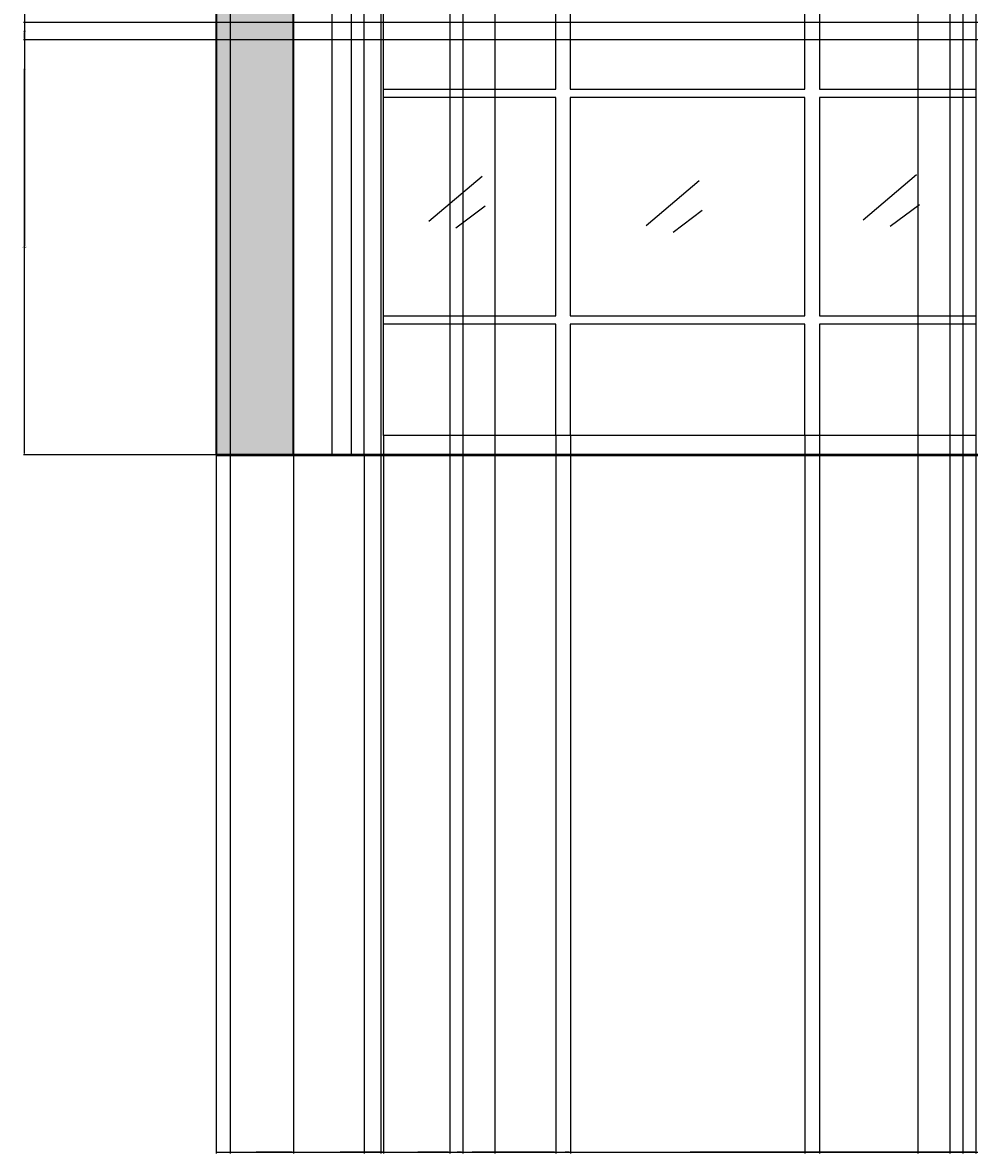
# Model space of a CAD drawing. Units: inches. Extents: x -13 to 630, y -103 to 275.
# Tile 1 of 9: x -13 to 134, y -103 to 72. Entities that reach past the tile are written whole.
import ezdxf

# ---------------------------------------------------------------- set-up
doc = ezdxf.new("R2010")
doc.units = ezdxf.units.IN
doc.header["$MEASUREMENT"] = 0
for name, color, linetype, lineweight in [('A-ANNO-DIMS', 2, 'Continuous', 18), ('A-ELEV', 7, 'Continuous', 35), ('A-ELEV-GRND', 7, 'Continuous', 50), ('A-ELEV-PATT', 8, 'Continuous', 13), ('A-GLAZ', 4, 'Continuous', 25)]:
    doc.layers.add(name, color=color, linetype=linetype, lineweight=lineweight)
doc.styles.get("Standard").update_dxf_attribs({"font": 'arial.ttf'})
doc.dimstyles.get("Standard").update_dxf_attribs({"dimtxt": 0.18, "dimasz": 0.18, "dimexe": 0.18, "dimexo": 0.0625, "dimgap": 0.09, "dimtad": 0, "dimtih": 1, "dimtoh": 1, "dimdec": 4, "dimzin": 0, "dimdsep": 46, "dimtxsty": 'Standard', "dimcen": 0.09, "dimadec": 0, "dimazin": 0, "dimtfac": 1, "dimtdec": 4, "dimtofl": 0, "dimtmove": 0, "dimatfit": 3, "dimfxl": 1, "dimtolj": 1, "dimtzin": 0, "dimarcsym": 0})

# ---------------------------------------------------------------- blocks, each defined once
blk = doc.blocks.new('WIN-GROUND')
for points in [[(0, 0), (0, 102), (108, 102), (108, 0)], [(3, 0), (3, 99), (105, 99), (105, 0)], [(5, 0), (5, 97), (103, 97), (103, 0)], [(34.74, 56.82), (34.74, 73.49), (37, 73.49), (37, 56.82)], [(73.43, 56.82), (73.43, 73.49), (75.7, 73.49), (75.7, 56.82)], [(34.74, 55.51), (8, 55.51), (8, 56.82), (34.74, 56.82)], [(37, 56.82), (73.43, 56.82)], [(75.7, 56.82), (100, 56.82), (100, 55.51), (75.7, 55.51)], [(34.74, 21.58), (34.74, 55.51)], [(37, 55.51), (37, 21.58)], [(73.43, 55.51), (37, 55.51)], [(73.43, 21.58), (73.43, 55.51)], [(75.7, 55.51), (75.7, 21.58)], [(34.74, 20.27), (8, 20.27), (8, 21.58), (34.74, 21.58)], [(37, 21.58), (73.43, 21.58)], [(75.7, 21.58), (100, 21.58), (100, 20.27), (75.7, 20.27)], [(37, 20.27), (37, 3), (34.74, 3), (34.74, 20.27)], [(73.43, 20.27), (37, 20.27)], [(75.7, 20.27), (75.7, 3), (73.43, 3), (73.43, 20.27)]]:
    blk.add_lwpolyline(points)
for points in [[(5, 97), (103, 97), (103, 76.49), (5, 76.49)], [(5, 76.49), (103, 76.49), (103, 0), (5, 0)], [(8, 73.49), (100, 73.49), (100, 3), (8, 3)]]:
    blk.add_lwpolyline(points, close=True)
blk = doc.blocks.new('GLAZ-MARK')
for p, q in [((0, 1.02), (8.26, 8.03)), ((4.19, 0), (8.71, 3.39))]:
    blk.add_line(p, q)
blk = doc.blocks.new('*D7')
at = {"layer": 'A-ANNO-DIMS', "color": 0, "lineweight": -2, "transparency": 16777216}
for p, q in [((16.71, 5.14), (16.71, 275.01)), ((16.89, 274.83), (25.5, 274.83)), ((34.53, 274.83), (25.92, 274.83)), ((34.71, 5.14), (34.71, 275.01))]:
    blk.add_line(p, q, dxfattribs=at)
at = {"layer": 'A-ANNO-DIMS', "color": 0, "transparency": 16777216}
for points in [[(16.89, 274.86), (16.89, 274.8), (16.71, 274.83)], [(34.53, 274.86), (34.53, 274.8), (34.71, 274.83)]]:
    blk.add_solid(points, dxfattribs=at)
at = {"layer": 'Defpoints', "color": 0, "transparency": 16777216}
for p in [(34.71, 274.83), (16.71, 5.08), (34.71, 5.08)]:
    blk.add_point(p, dxfattribs=at)
at = {"layer": 'A-ANNO-DIMS', "color": 0, "transparency": 16777216, "insert": (25.71, 274.83), "char_height": 0.18, "attachment_point": 5}
blk.add_mtext('\\A1;18', dxfattribs=at)
blk = doc.blocks.new('*D11')
at = {"layer": 'A-ANNO-DIMS', "color": 0, "lineweight": -2, "transparency": 16777216}
for p, q in [((16.71, 5.02), (16.71, -103.45)), ((496.71, 5.02), (496.71, -103.45)), ((16.89, -103.27), (256.42, -103.27)), ((496.53, -103.27), (257, -103.27))]:
    blk.add_line(p, q, dxfattribs=at)
at = {"layer": 'A-ANNO-DIMS', "color": 0, "transparency": 16777216}
for points in [[(16.89, -103.24), (16.89, -103.3), (16.71, -103.27)], [(496.53, -103.24), (496.53, -103.3), (496.71, -103.27)]]:
    blk.add_solid(points, dxfattribs=at)
at = {"layer": 'Defpoints', "color": 0, "transparency": 16777216}
for p in [(16.71, 5.08), (496.71, 5.08), (496.71, -103.27)]:
    blk.add_point(p, dxfattribs=at)
at = {"layer": 'A-ANNO-DIMS', "color": 0, "transparency": 16777216, "insert": (256.71, -103.27), "char_height": 0.18, "attachment_point": 5}
blk.add_mtext('\\A1;480', dxfattribs=at)
blk = doc.blocks.new('*D12')
at = {"layer": 'A-ANNO-DIMS', "color": 0, "lineweight": -2, "transparency": 16777216}
for p, q in [((16.65, 125.08), (-13.22, 125.08)), ((-13.04, 124.9), (-13.04, 65.26)), ((-13.04, 5.26), (-13.04, 64.9)), ((16.65, 5.08), (-13.22, 5.08))]:
    blk.add_line(p, q, dxfattribs=at)
at = {"layer": 'A-ANNO-DIMS', "color": 0, "transparency": 16777216}
for points in [[(-13.07, 124.9), (-13.01, 124.9), (-13.04, 125.08)], [(-13.07, 5.26), (-13.01, 5.26), (-13.04, 5.08)]]:
    blk.add_solid(points, dxfattribs=at)
at = {"layer": 'Defpoints', "color": 0, "transparency": 16777216}
for p in [(-13.04, 125.08), (16.71, 125.08), (16.71, 5.08)]:
    blk.add_point(p, dxfattribs=at)
at = {"layer": 'A-ANNO-DIMS', "color": 0, "transparency": 16777216, "insert": (-13.04, 65.08), "char_height": 0.18, "attachment_point": 5}
blk.add_mtext('\\A1;120', dxfattribs=at)
blk = doc.blocks.new('*D40')
at = {"layer": 'A-ANNO-DIMS', "color": 0, "lineweight": -2, "transparency": 16777216}
for p, q in [((205.96, 69.55), (-13.22, 69.55)), ((-13.04, 69.37), (-13.04, 37.5)), ((-13.04, 5.26), (-13.04, 37.13)), ((205.96, 5.08), (-13.22, 5.08))]:
    blk.add_line(p, q, dxfattribs=at)
at = {"layer": 'A-ANNO-DIMS', "color": 0, "transparency": 16777216}
for points in [[(-13.07, 69.37), (-13.01, 69.37), (-13.04, 69.55)], [(-13.07, 5.26), (-13.01, 5.26), (-13.04, 5.08)]]:
    blk.add_solid(points, dxfattribs=at)
at = {"layer": 'Defpoints', "color": 0, "transparency": 16777216}
for p in [(-13.04, 69.55), (206.02, 69.55), (206.02, 5.08)]:
    blk.add_point(p, dxfattribs=at)
at = {"layer": 'A-ANNO-DIMS', "color": 0, "transparency": 16777216, "insert": (-13.04, 37.31), "char_height": 0.18, "attachment_point": 5}
blk.add_mtext('\\A1;64.46', dxfattribs=at)
blk = doc.blocks.new('*D41')
at = {"layer": 'A-ANNO-DIMS', "color": 0, "lineweight": -2, "transparency": 16777216}
for p, q in [((205.96, 72.22), (-13.22, 72.22)), ((-13.04, 72.04), (-13.04, 71.07)), ((-13.04, 69.73), (-13.04, 70.7)), ((205.96, 69.55), (-13.22, 69.55))]:
    blk.add_line(p, q, dxfattribs=at)
at = {"layer": 'A-ANNO-DIMS', "color": 0, "transparency": 16777216}
for points in [[(-13.07, 72.04), (-13.01, 72.04), (-13.04, 72.22)], [(-13.07, 69.73), (-13.01, 69.73), (-13.04, 69.55)]]:
    blk.add_solid(points, dxfattribs=at)
at = {"layer": 'Defpoints', "color": 0, "transparency": 16777216}
for p in [(-13.04, 72.22), (206.02, 72.22), (206.02, 69.55)]:
    blk.add_point(p, dxfattribs=at)
at = {"layer": 'A-ANNO-DIMS', "color": 0, "transparency": 16777216, "insert": (-13.04, 70.88), "char_height": 0.18, "attachment_point": 5}
blk.add_mtext('\\A1;2.68', dxfattribs=at)
blk = doc.blocks.new('*D71')
at = {"layer": 'A-ANNO-DIMS', "color": 0, "lineweight": -2, "transparency": 16777216}
for p, q in [((42.71, 8.02), (42.71, -103.45)), ((39.71, 5.02), (39.71, -103.45)), ((39.89, -103.27), (41.06, -103.27)), ((42.53, -103.27), (41.36, -103.27))]:
    blk.add_line(p, q, dxfattribs=at)
at = {"layer": 'A-ANNO-DIMS', "color": 0, "transparency": 16777216}
for points in [[(39.89, -103.24), (39.89, -103.3), (39.71, -103.27)], [(42.53, -103.24), (42.53, -103.3), (42.71, -103.27)]]:
    blk.add_solid(points, dxfattribs=at)
at = {"layer": 'Defpoints', "color": 0, "transparency": 16777216}
for p in [(42.71, 8.08), (39.71, 5.08), (42.71, -103.27)]:
    blk.add_point(p, dxfattribs=at)
at = {"layer": 'A-ANNO-DIMS', "color": 0, "transparency": 16777216, "insert": (41.21, -103.27), "char_height": 0.18, "attachment_point": 5}
blk.add_mtext('\\A1;3', dxfattribs=at)
blk = doc.blocks.new('*D72')
at = {"layer": 'A-ANNO-DIMS', "color": 0, "lineweight": -2, "transparency": 16777216}
for p, q in [((42.71, 8.02), (42.71, -103.45)), ((69.45, 8.02), (69.45, -103.45)), ((42.89, -103.27), (55.69, -103.27)), ((69.27, -103.27), (56.48, -103.27))]:
    blk.add_line(p, q, dxfattribs=at)
at = {"layer": 'A-ANNO-DIMS', "color": 0, "transparency": 16777216}
for points in [[(42.89, -103.24), (42.89, -103.3), (42.71, -103.27)], [(69.27, -103.24), (69.27, -103.3), (69.45, -103.27)]]:
    blk.add_solid(points, dxfattribs=at)
at = {"layer": 'Defpoints', "color": 0, "transparency": 16777216}
for p in [(42.71, 8.08), (69.45, 8.08), (69.45, -103.27)]:
    blk.add_point(p, dxfattribs=at)
at = {"layer": 'A-ANNO-DIMS', "color": 0, "transparency": 16777216, "insert": (56.08, -103.27), "char_height": 0.18, "attachment_point": 5}
blk.add_mtext('\\A1;26.74', dxfattribs=at)
blk = doc.blocks.new('*D73')
at = {"layer": 'A-ANNO-DIMS', "color": 0, "lineweight": -2, "transparency": 16777216}
for p, q in [((69.45, 8.02), (69.45, -103.45)), ((71.72, 8.02), (71.72, -103.45)), ((69.63, -103.27), (70.26, -103.27)), ((71.54, -103.27), (70.91, -103.27))]:
    blk.add_line(p, q, dxfattribs=at)
at = {"layer": 'A-ANNO-DIMS', "color": 0, "transparency": 16777216}
for points in [[(69.63, -103.24), (69.63, -103.3), (69.45, -103.27)], [(71.54, -103.24), (71.54, -103.3), (71.72, -103.27)]]:
    blk.add_solid(points, dxfattribs=at)
at = {"layer": 'Defpoints', "color": 0, "transparency": 16777216}
for p in [(69.45, 8.08), (71.72, 8.08), (71.72, -103.27)]:
    blk.add_point(p, dxfattribs=at)
at = {"layer": 'A-ANNO-DIMS', "color": 0, "transparency": 16777216, "insert": (70.58, -103.27), "char_height": 0.18, "attachment_point": 5}
blk.add_mtext('\\A1;2.27', dxfattribs=at)
blk = doc.blocks.new('*D74')
at = {"layer": 'A-ANNO-DIMS', "color": 0, "lineweight": -2, "transparency": 16777216}
for p, q in [((71.72, 8.02), (71.72, -103.45)), ((108.15, 8.02), (108.15, -103.45)), ((71.9, -103.27), (89.54, -103.27)), ((107.97, -103.27), (90.32, -103.27))]:
    blk.add_line(p, q, dxfattribs=at)
at = {"layer": 'A-ANNO-DIMS', "color": 0, "transparency": 16777216}
for points in [[(71.9, -103.24), (71.9, -103.3), (71.72, -103.27)], [(107.97, -103.24), (107.97, -103.3), (108.15, -103.27)]]:
    blk.add_solid(points, dxfattribs=at)
at = {"layer": 'Defpoints', "color": 0, "transparency": 16777216}
for p in [(71.72, 8.08), (108.15, 8.08), (108.15, -103.27)]:
    blk.add_point(p, dxfattribs=at)
at = {"layer": 'A-ANNO-DIMS', "color": 0, "transparency": 16777216, "insert": (89.93, -103.27), "char_height": 0.18, "attachment_point": 5}
blk.add_mtext('\\A1;36.43', dxfattribs=at)
blk = doc.blocks.new('*D75')
at = {"layer": 'A-ANNO-DIMS', "color": 0, "lineweight": -2, "transparency": 16777216}
for p, q in [((108.15, 8.02), (108.15, -103.45)), ((110.41, 8.02), (110.41, -103.45)), ((108.33, -103.27), (108.95, -103.27)), ((110.23, -103.27), (109.6, -103.27))]:
    blk.add_line(p, q, dxfattribs=at)
at = {"layer": 'A-ANNO-DIMS', "color": 0, "transparency": 16777216}
for points in [[(108.33, -103.24), (108.33, -103.3), (108.15, -103.27)], [(110.23, -103.24), (110.23, -103.3), (110.41, -103.27)]]:
    blk.add_solid(points, dxfattribs=at)
at = {"layer": 'Defpoints', "color": 0, "transparency": 16777216}
for p in [(108.15, 8.08), (110.41, 8.08), (110.41, -103.27)]:
    blk.add_point(p, dxfattribs=at)
at = {"layer": 'A-ANNO-DIMS', "color": 0, "transparency": 16777216, "insert": (109.28, -103.27), "char_height": 0.18, "attachment_point": 5}
blk.add_mtext('\\A1;2.27', dxfattribs=at)
blk = doc.blocks.new('*D76')
at = {"layer": 'A-ANNO-DIMS', "color": 0, "lineweight": -2, "transparency": 16777216}
for p, q in [((110.41, 8.02), (110.41, -103.45)), ((134.71, 8.02), (134.71, -103.45)), ((110.59, -103.27), (122.24, -103.27)), ((134.53, -103.27), (122.89, -103.27))]:
    blk.add_line(p, q, dxfattribs=at)
at = {"layer": 'A-ANNO-DIMS', "color": 0, "transparency": 16777216}
for points in [[(110.59, -103.24), (110.59, -103.3), (110.41, -103.27)], [(134.53, -103.24), (134.53, -103.3), (134.71, -103.27)]]:
    blk.add_solid(points, dxfattribs=at)
at = {"layer": 'Defpoints', "color": 0, "transparency": 16777216}
for p in [(110.41, 8.08), (134.71, 8.08), (134.71, -103.27)]:
    blk.add_point(p, dxfattribs=at)
at = {"layer": 'A-ANNO-DIMS', "color": 0, "transparency": 16777216, "insert": (122.56, -103.27), "char_height": 0.18, "attachment_point": 5}
blk.add_mtext('\\A1;24.3', dxfattribs=at)
blk = doc.blocks.new('*D103')
at = {"layer": 'A-ANNO-DIMS', "color": 0, "lineweight": -2, "transparency": 16777216}
for p, q in [((18.87, 197.26), (18.87, -103.45)), ((28.71, 197.26), (28.71, -103.45)), ((19.05, -103.27), (23.4, -103.27)), ((28.53, -103.27), (24.19, -103.27))]:
    blk.add_line(p, q, dxfattribs=at)
at = {"layer": 'A-ANNO-DIMS', "color": 0, "transparency": 16777216}
for points in [[(19.05, -103.24), (19.05, -103.3), (18.87, -103.27)], [(28.53, -103.24), (28.53, -103.3), (28.71, -103.27)]]:
    blk.add_solid(points, dxfattribs=at)
at = {"layer": 'Defpoints', "color": 0, "transparency": 16777216}
for p in [(18.87, 197.32), (28.71, 197.32), (28.71, -103.27)]:
    blk.add_point(p, dxfattribs=at)
at = {"layer": 'A-ANNO-DIMS', "color": 0, "transparency": 16777216, "insert": (23.79, -103.27), "char_height": 0.18, "attachment_point": 5}
blk.add_mtext('\\A1;9.838', dxfattribs=at)
blk = doc.blocks.new('*D104')
at = {"layer": 'A-ANNO-DIMS', "color": 0, "lineweight": -2, "transparency": 16777216}
for p, q in [((16.71, 125.02), (16.71, -103.45)), ((28.71, 125.02), (28.71, -103.45)), ((16.89, -103.27), (22.5, -103.27)), ((28.53, -103.27), (22.92, -103.27))]:
    blk.add_line(p, q, dxfattribs=at)
at = {"layer": 'A-ANNO-DIMS', "color": 0, "transparency": 16777216}
for points in [[(16.89, -103.24), (16.89, -103.3), (16.71, -103.27)], [(28.53, -103.24), (28.53, -103.3), (28.71, -103.27)]]:
    blk.add_solid(points, dxfattribs=at)
at = {"layer": 'Defpoints', "color": 0, "transparency": 16777216}
for p in [(16.71, 125.08), (28.71, 125.08), (28.71, -103.27)]:
    blk.add_point(p, dxfattribs=at)
at = {"layer": 'A-ANNO-DIMS', "color": 0, "transparency": 16777216, "insert": (22.71, -103.27), "char_height": 0.18, "attachment_point": 5}
blk.add_mtext('\\A1;12', dxfattribs=at)
blk = doc.blocks.new('*D105')
at = {"layer": 'A-ANNO-DIMS', "color": 0, "lineweight": -2, "transparency": 16777216}
for p, q in [((28.71, 125.02), (28.71, -103.45)), ((42.29, 125.02), (42.29, -103.45)), ((28.89, -103.27), (35.04, -103.27)), ((42.11, -103.27), (35.95, -103.27))]:
    blk.add_line(p, q, dxfattribs=at)
at = {"layer": 'A-ANNO-DIMS', "color": 0, "transparency": 16777216}
for points in [[(28.89, -103.24), (28.89, -103.3), (28.71, -103.27)], [(42.11, -103.24), (42.11, -103.3), (42.29, -103.27)]]:
    blk.add_solid(points, dxfattribs=at)
at = {"layer": 'Defpoints', "color": 0, "transparency": 16777216}
for p in [(28.71, 125.08), (42.29, 125.08), (42.29, -103.27)]:
    blk.add_point(p, dxfattribs=at)
at = {"layer": 'A-ANNO-DIMS', "color": 0, "transparency": 16777216, "insert": (35.5, -103.27), "char_height": 0.18, "attachment_point": 5}
blk.add_mtext('\\A1;13.574', dxfattribs=at)
blk = doc.blocks.new('*D106')
at = {"layer": 'A-ANNO-DIMS', "color": 0, "lineweight": -2, "transparency": 16777216}
for p, q in [((42.29, 125.02), (42.29, -103.45)), ((53, 125.02), (53, -103.45)), ((42.47, -103.27), (47.27, -103.27)), ((52.82, -103.27), (48.01, -103.27))]:
    blk.add_line(p, q, dxfattribs=at)
at = {"layer": 'A-ANNO-DIMS', "color": 0, "transparency": 16777216}
for points in [[(42.47, -103.24), (42.47, -103.3), (42.29, -103.27)], [(52.82, -103.24), (52.82, -103.3), (53, -103.27)]]:
    blk.add_solid(points, dxfattribs=at)
at = {"layer": 'Defpoints', "color": 0, "transparency": 16777216}
for p in [(42.29, 125.08), (53, 125.08), (53, -103.27)]:
    blk.add_point(p, dxfattribs=at)
at = {"layer": 'A-ANNO-DIMS', "color": 0, "transparency": 16777216, "insert": (47.64, -103.27), "char_height": 0.18, "attachment_point": 5}
blk.add_mtext('\\A1;10.71', dxfattribs=at)
blk = doc.blocks.new('*D107')
at = {"layer": 'A-ANNO-DIMS', "color": 0, "lineweight": -2, "transparency": 16777216}
for p, q in [((53, 125.02), (53, -103.45)), ((55, 125.02), (55, -103.45)), ((53.18, -103.27), (53.85, -103.27)), ((54.82, -103.27), (54.14, -103.27))]:
    blk.add_line(p, q, dxfattribs=at)
at = {"layer": 'A-ANNO-DIMS', "color": 0, "transparency": 16777216}
for points in [[(53.18, -103.24), (53.18, -103.3), (53, -103.27)], [(54.82, -103.24), (54.82, -103.3), (55, -103.27)]]:
    blk.add_solid(points, dxfattribs=at)
at = {"layer": 'Defpoints', "color": 0, "transparency": 16777216}
for p in [(53, 125.08), (55, 125.08), (55, -103.27)]:
    blk.add_point(p, dxfattribs=at)
at = {"layer": 'A-ANNO-DIMS', "color": 0, "transparency": 16777216, "insert": (54, -103.27), "char_height": 0.18, "attachment_point": 5}
blk.add_mtext('\\A1;2', dxfattribs=at)
blk = doc.blocks.new('*D108')
at = {"layer": 'A-ANNO-DIMS', "color": 0, "lineweight": -2, "transparency": 16777216}
for p, q in [((55, 125.02), (55, -103.45)), ((60, 125.02), (60, -103.45)), ((55.18, -103.27), (57.35, -103.27)), ((59.82, -103.27), (57.64, -103.27))]:
    blk.add_line(p, q, dxfattribs=at)
at = {"layer": 'A-ANNO-DIMS', "color": 0, "transparency": 16777216}
for points in [[(55.18, -103.24), (55.18, -103.3), (55, -103.27)], [(59.82, -103.24), (59.82, -103.3), (60, -103.27)]]:
    blk.add_solid(points, dxfattribs=at)
at = {"layer": 'Defpoints', "color": 0, "transparency": 16777216}
for p in [(55, 125.08), (60, 125.08), (60, -103.27)]:
    blk.add_point(p, dxfattribs=at)
at = {"layer": 'A-ANNO-DIMS', "color": 0, "transparency": 16777216, "insert": (57.5, -103.27), "char_height": 0.18, "attachment_point": 5}
blk.add_mtext('\\A1;5', dxfattribs=at)
blk = doc.blocks.new('*D109')
at = {"layer": 'A-ANNO-DIMS', "color": 0, "lineweight": -2, "transparency": 16777216}
for p, q in [((60, 125.02), (60, -103.45)), ((125.66, 125.02), (125.66, -103.45)), ((60.18, -103.27), (92.44, -103.27)), ((125.48, -103.27), (93.22, -103.27))]:
    blk.add_line(p, q, dxfattribs=at)
at = {"layer": 'A-ANNO-DIMS', "color": 0, "transparency": 16777216}
for points in [[(60.18, -103.24), (60.18, -103.3), (60, -103.27)], [(125.48, -103.24), (125.48, -103.3), (125.66, -103.27)]]:
    blk.add_solid(points, dxfattribs=at)
at = {"layer": 'Defpoints', "color": 0, "transparency": 16777216}
for p in [(60, 125.08), (125.66, 125.08), (125.66, -103.27)]:
    blk.add_point(p, dxfattribs=at)
at = {"layer": 'A-ANNO-DIMS', "color": 0, "transparency": 16777216, "insert": (92.83, -103.27), "char_height": 0.18, "attachment_point": 5}
blk.add_mtext('\\A1;65.67', dxfattribs=at)
blk = doc.blocks.new('*D110')
at = {"layer": 'A-ANNO-DIMS', "color": 0, "lineweight": -2, "transparency": 16777216}
for p, q in [((125.66, 125.02), (125.66, -103.45)), ((130.66, 125.02), (130.66, -103.45)), ((125.84, -103.27), (128.01, -103.27)), ((130.48, -103.27), (128.31, -103.27))]:
    blk.add_line(p, q, dxfattribs=at)
at = {"layer": 'A-ANNO-DIMS', "color": 0, "transparency": 16777216}
for points in [[(125.84, -103.24), (125.84, -103.3), (125.66, -103.27)], [(130.48, -103.24), (130.48, -103.3), (130.66, -103.27)]]:
    blk.add_solid(points, dxfattribs=at)
at = {"layer": 'Defpoints', "color": 0, "transparency": 16777216}
for p in [(125.66, 125.08), (130.66, 125.08), (130.66, -103.27)]:
    blk.add_point(p, dxfattribs=at)
at = {"layer": 'A-ANNO-DIMS', "color": 0, "transparency": 16777216, "insert": (128.16, -103.27), "char_height": 0.18, "attachment_point": 5}
blk.add_mtext('\\A1;5', dxfattribs=at)
blk = doc.blocks.new('*D111')
at = {"layer": 'A-ANNO-DIMS', "color": 0, "lineweight": -2, "transparency": 16777216}
for p, q in [((130.66, 125.02), (130.66, -103.45)), ((132.66, 125.02), (132.66, -103.45)), ((130.84, -103.27), (131.51, -103.27)), ((132.48, -103.27), (131.81, -103.27))]:
    blk.add_line(p, q, dxfattribs=at)
at = {"layer": 'A-ANNO-DIMS', "color": 0, "transparency": 16777216}
for points in [[(130.84, -103.24), (130.84, -103.3), (130.66, -103.27)], [(132.48, -103.24), (132.48, -103.3), (132.66, -103.27)]]:
    blk.add_solid(points, dxfattribs=at)
at = {"layer": 'Defpoints', "color": 0, "transparency": 16777216}
for p in [(130.66, 125.08), (132.66, 125.08), (132.66, -103.27)]:
    blk.add_point(p, dxfattribs=at)
at = {"layer": 'A-ANNO-DIMS', "color": 0, "transparency": 16777216, "insert": (131.66, -103.27), "char_height": 0.18, "attachment_point": 5}
blk.add_mtext('\\A1;2', dxfattribs=at)
blk = doc.blocks.new('*D112')
at = {"layer": 'A-ANNO-DIMS', "color": 0, "lineweight": -2, "transparency": 16777216}
for p, q in [((132.66, 125.02), (132.66, -103.45)), ((164.84, 125.02), (164.84, -103.45)), ((132.84, -103.27), (148.36, -103.27)), ((164.66, -103.27), (149.15, -103.27))]:
    blk.add_line(p, q, dxfattribs=at)
at = {"layer": 'A-ANNO-DIMS', "color": 0, "transparency": 16777216}
for points in [[(132.84, -103.24), (132.84, -103.3), (132.66, -103.27)], [(164.66, -103.24), (164.66, -103.3), (164.84, -103.27)]]:
    blk.add_solid(points, dxfattribs=at)
at = {"layer": 'Defpoints', "color": 0, "transparency": 16777216}
for p in [(132.66, 125.08), (164.84, 125.08), (164.84, -103.27)]:
    blk.add_point(p, dxfattribs=at)
at = {"layer": 'A-ANNO-DIMS', "color": 0, "transparency": 16777216, "insert": (148.75, -103.27), "char_height": 0.18, "attachment_point": 5}
blk.add_mtext('\\A1;32.18', dxfattribs=at)

msp = doc.modelspace()

# ---------------------------------------------------------------- hatches: boundary and pattern name
at = {"layer": 'A-ELEV-PATT'}
h = msp.add_hatch(dxfattribs=at)
h.set_pattern_fill('BRSTONE', color=256, scale=20)
h.paths.add_polyline_path([(120.6641, 172.7854), (64.9953, 172.7854, 0.41421356), (54.9953, 162.7854), (54.9953, 125.0808), (59.9953, 125.0808), (59.9953, 162.7854, -0.41421356), (64.9953, 167.7854), (120.6641, 167.7854, -0.41421356), (125.6641, 162.7854), (125.6641, 125.0808), (130.6641, 125.0808), (130.6641, 162.7854, 0.41421356)])
h.paths.add_polyline_path([(439.5513, 172.7854), (383.8825, 172.7854, 0.41421356), (373.8825, 162.7854), (373.8825, 125.0808), (378.8825, 125.0808), (378.8825, 162.7854, -0.41421356), (383.8825, 167.7854), (439.5513, 167.7854, -0.41421356), (444.5513, 162.7854), (444.5513, 125.0808), (449.5513, 125.0808), (449.5513, 162.7854, 0.41421356)])
h.paths.add_polyline_path([(364.7117, 113.0808), (484.7117, 113.0808), (484.7117, 5.0808), (496.7117, 5.0808), (496.7117, 125.0808), (345.3061, 125.0808), (345.3061, 5.0808), (364.7117, 5.0808)])
h.paths.add_polyline_path([(164.8443, 125.0808), (28.7117, 125.0808), (16.7117, 125.0808), (16.7117, 5.0808), (28.7117, 5.0808), (28.7117, 113.0808), (148.7117, 113.0808), (148.7117, 5.0808), (164.8443, 5.0808)])
h.paths.add_polyline_path([(95.1171, 223.9392), (83.8622, 223.9392), (83.8622, 206.5279), (95.1171, 206.5279)])
h.paths.add_polyline_path([(54.9212, 223.9392), (40.7186, 223.9392), (40.7186, 206.5279), (54.9212, 206.5279)])
h.paths.add_polyline_path([(463.828, 223.9392), (449.6254, 223.9392), (449.6254, 206.5279), (463.828, 206.5279)])
h.paths.add_polyline_path([(420.6843, 223.9392), (409.4295, 223.9392), (409.4295, 206.5279), (420.6843, 206.5279)])

# ---------------------------------------------------------------- linework, layer by layer
at = {"layer": 'A-ELEV'}
for points in [[(164.8443, 125.0808), (16.7117, 125.0808), (16.7117, 5.0808)], [(28.7117, 5.0808), (28.7117, 113.0808), (148.7117, 113.0808), (148.7117, 5.0808)]]:
    msp.add_lwpolyline(points, dxfattribs=at)
at = {"layer": 'A-ELEV-GRND'}
msp.add_line((16.7117, 5.0808), (496.7117, 5.0808), dxfattribs=at)

# ---------------------------------------------------------------- block references
at = {"layer": 'A-GLAZ'}
for name, p in [('WIN-GROUND', (34.712, 5.081)), ('GLAZ-MARK', (49.7536, 40.3504)), ('GLAZ-MARK', (83.481, 39.672)), ('GLAZ-MARK', (117.2084, 40.5766))]:
    msp.add_blockref(name, p, dxfattribs=at)

# ---------------------------------------------------------------- dimensions: what is measured, and where the dimension line sits
at = {"layer": 'A-ANNO-DIMS'}
for base, p1, p2, override, picture, middle in [((34.7117, 274.8308), (16.7117, 5.0808), (34.7117, 5.0808), {"dimdec": 0, "dimlfac": 1, "dimrnd": 0, "dimzin": 0, "dimdsep": 46, "dimlunit": 2}, '*D7', (25.7117, 274.8308)), ((28.71172, -103.27457), (18.87325, 197.32155), (28.71172, 197.32155), {"dimdec": 3, "dimlfac": 1, "dimrnd": 0, "dimzin": 0, "dimdsep": 46, "dimlunit": 2}, '*D103', (23.79248, -103.27457)), ((28.7117, -103.2746), (16.7117, 125.0808), (28.7117, 125.0808), {"dimdec": 0, "dimlfac": 1, "dimrnd": 0, "dimzin": 0, "dimdsep": 46, "dimlunit": 2}, '*D104', (22.7117, -103.2746)), ((42.2856, -103.2746), (28.7117, 125.0808), (42.2856, 125.0808), {"dimdec": 3, "dimlfac": 1, "dimrnd": 0, "dimzin": 0, "dimdsep": 46, "dimlunit": 2}, '*D105', (35.4987, -103.2746)), ((52.9953, -103.2746), (42.2856, 125.0808), (52.9953, 125.0808), {"dimdec": 2, "dimlfac": 1, "dimrnd": 0, "dimzin": 0, "dimdsep": 46, "dimlunit": 2}, '*D106', (47.6404, -103.2746)), ((54.9953, -103.2746), (52.9953, 125.0808), (54.9953, 125.0808), {"dimdec": 0, "dimlfac": 1, "dimrnd": 0, "dimzin": 0, "dimdsep": 46, "dimlunit": 2}, '*D107', (53.9953, -103.2746)), ((59.9953, -103.2746), (54.9953, 125.0808), (59.9953, 125.0808), {"dimdec": 0, "dimlfac": 1, "dimrnd": 0, "dimzin": 0, "dimdsep": 46, "dimlunit": 2}, '*D108', (57.4953, -103.2746)), ((125.6641, -103.2746), (59.9953, 125.0808), (125.6641, 125.0808), {"dimdec": 2, "dimlfac": 1, "dimrnd": 0, "dimzin": 0, "dimdsep": 46, "dimlunit": 2}, '*D109', (92.8297, -103.2746)), ((130.6641, -103.2746), (125.6641, 125.0808), (130.6641, 125.0808), {"dimdec": 0, "dimlfac": 1, "dimrnd": 0, "dimzin": 0, "dimdsep": 46, "dimlunit": 2}, '*D110', (128.1641, -103.2746)), ((132.6641, -103.2746), (130.6641, 125.0808), (132.6641, 125.0808), {"dimdec": 0, "dimlfac": 1, "dimrnd": 0, "dimzin": 0, "dimdsep": 46, "dimlunit": 2}, '*D111', (131.6641, -103.2746)), ((164.8443, -103.2746), (132.6641, 125.0808), (164.8443, 125.0808), {"dimdec": 2, "dimlfac": 1, "dimrnd": 0, "dimzin": 0, "dimdsep": 46, "dimlunit": 2}, '*D112', (148.7542, -103.2746)), ((42.7117, -103.2746), (39.7117, 5.0808), (42.7117, 8.0808), {"dimdec": 0, "dimlfac": 1, "dimrnd": 0, "dimzin": 0, "dimdsep": 46, "dimlunit": 2}, '*D71', (41.2117, -103.2746)), ((69.4498, -103.2746), (42.7117, 8.0808), (69.4498, 8.0808), {"dimdec": 2, "dimlfac": 1, "dimrnd": 0, "dimzin": 0, "dimdsep": 46, "dimlunit": 2}, '*D72', (56.0808, -103.2746)), ((71.7162, -103.2746), (69.4498, 8.0808), (71.7162, 8.0808), {"dimdec": 2, "dimlfac": 1, "dimrnd": 0, "dimzin": 0, "dimdsep": 46, "dimlunit": 2}, '*D73', (70.583, -103.2746)), ((108.1459, -103.2746), (71.7162, 8.0808), (108.1459, 8.0808), {"dimdec": 2, "dimlfac": 1, "dimrnd": 0, "dimzin": 0, "dimdsep": 46, "dimlunit": 2}, '*D74', (89.931, -103.2746)), ((110.4122, -103.2746), (108.1459, 8.0808), (110.4122, 8.0808), {"dimdec": 2, "dimlfac": 1, "dimrnd": 0, "dimzin": 0, "dimdsep": 46, "dimlunit": 2}, '*D75', (109.2791, -103.2746)), ((134.7117, -103.2746), (110.4122, 8.0808), (134.7117, 8.0808), {"dimdec": 1, "dimlfac": 1, "dimrnd": 0, "dimzin": 0, "dimdsep": 46, "dimlunit": 2}, '*D76', (122.562, -103.2746)), ((496.7117, -103.2746), (16.7117, 5.0808), (496.7117, 5.0808), {"dimdec": 0, "dimlfac": 1, "dimrnd": 0, "dimzin": 0, "dimdsep": 46, "dimlunit": 2}, '*D11', (256.7117, -103.2746))]:
    dim = msp.add_linear_dim(base=base, p1=p1, p2=p2, dimstyle='Standard', override=override, dxfattribs=at)
    dim.commit()
    dim.dimension.update_dxf_attribs({"geometry": picture, "text_midpoint": middle})
for base, p1, p2, override, picture, middle in [((-13.0383, 125.0808), (16.7117, 5.0808), (16.7117, 125.0808), {"dimdec": 0, "dimlfac": 1, "dimrnd": 0, "dimzin": 0, "dimdsep": 46, "dimlunit": 2}, '*D12', (-13.0383, 65.0808)), ((-13.0383, 72.223), (206.0208, 69.5455), (206.0208, 72.223), {"dimdec": 2, "dimlfac": 1, "dimrnd": 0, "dimzin": 0, "dimdsep": 46, "dimlunit": 2}, '*D41', (-13.0383, 70.8842)), ((-13.0383, 69.5455), (206.0208, 5.0808), (206.0208, 69.5455), {"dimdec": 2, "dimlfac": 1, "dimrnd": 0, "dimzin": 0, "dimdsep": 46, "dimlunit": 2}, '*D40', (-13.0383, 37.3131))]:
    dim = msp.add_linear_dim(base=base, p1=p1, p2=p2, angle=90, dimstyle='Standard', override=override, dxfattribs=at)
    dim.commit()
    dim.dimension.update_dxf_attribs({"geometry": picture, "text_midpoint": middle})

doc.saveas('drawing.dxf')
